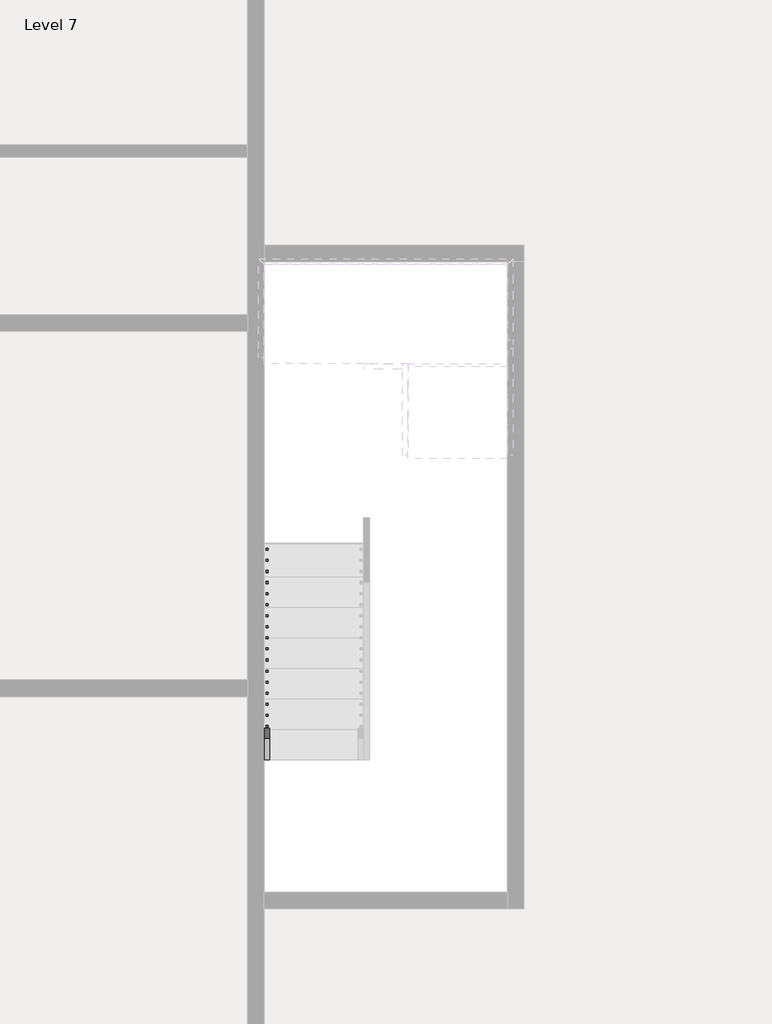
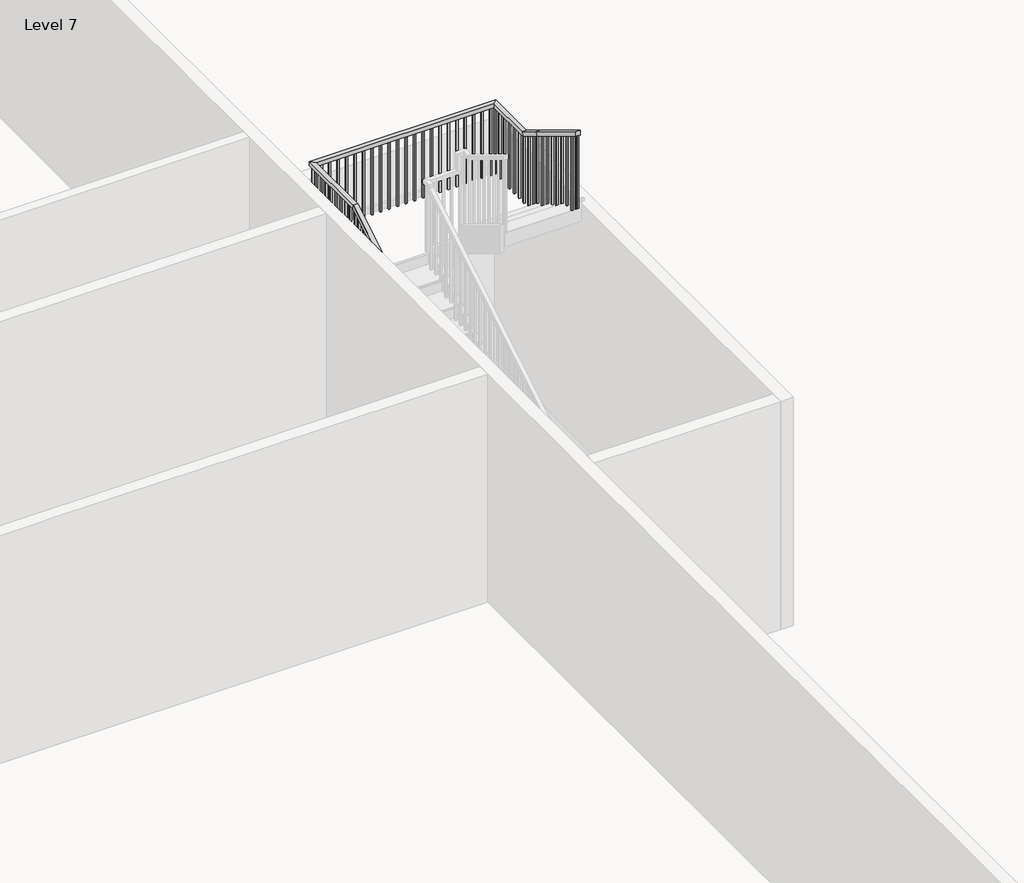
# One storey, part 6 of 8: 1 railing.
"""IFC4 building model written with IfcOpenShell, lengths in millimetres."""

from ifc_helpers import new_model, si_unit, frame, origin, place, context, project, spatial, polyline, outline, extrude, faceted_brep, element, save

model = new_model("IFC4")

# Units and contexts
model_context = context("Model", 3, world=origin())
ifc_project = project(units=[si_unit("LENGTHUNIT", "METRE", prefix="MILLI")], contexts=[model_context])

# Site, building, storey
site = spatial("IfcSite", under=ifc_project)
building = spatial("IfcBuilding", under=site)
storey = spatial("IfcBuildingStorey", under=building, Name="Level 7", Elevation=43522.6172466)

# Railing
placement = place(None, origin())
element("IfcRailing", 1, ObjectType="Handrail - Rectangular", at=placement, inside=storey, context=model_context, shape_type="SolidModel", body=[
    faceted_brep([(-3617.4415084, -23154.3851539, 44606.3505799), (-3617.4415084, -23154.3851539, 44546.9491197), (-3566.6415084, -23154.3851539, 44546.9491197), (-3566.6415084, -23154.3851539, 44606.3505799), (-3617.4415084, -19522.1851539, 46807.6839133), (-3617.4415084, -19507.9927445, 46756.8839133), (-3566.6415084, -19507.9927445, 46756.8839133), (-3566.6415084, -19522.1851539, 46807.6839133), (-3617.4415084, -18607.7851539, 46807.6839133), (-3617.4415084, -18607.7851539, 46756.8839133), (-3566.6415084, -18658.5851539, 46756.8839133), (-3566.6415084, -18658.5851539, 46807.6839133), (-1382.2415084, -18607.7851539, 46807.6839133), (-1382.2415084, -18607.7851539, 46756.8839133), (-1433.0415084, -18658.5851539, 46756.8839133), (-1433.0415084, -18658.5851539, 46807.6839133), (-1382.2415084, -19242.7851539, 46807.6839133), (-1382.2415084, -19256.9775633, 46756.8839133), (-1433.0415084, -19256.9775633, 46756.8839133), (-1433.0415084, -19242.7851539, 46807.6839133), (-1382.2415084, -19522.1851539, 46977.0172466), (-1382.2415084, -19548.5148811, 46933.5731968), (-1433.0415084, -19548.5148811, 46933.5731968), (-1433.0415084, -19522.1851539, 46977.0172466), (-1382.2415084, -20360.3851539, 47485.0172466), (-1433.0415084, -20360.3851539, 47485.0172466), (-1433.0415084, -20360.3851539, 47425.6157863), (-1382.2415084, -20360.3851539, 47425.6157863)], [[[0, 1, 2, 3]], [[1, 0, 4, 5]], [[2, 1, 5, 6]], [[3, 2, 6, 7]], [[0, 3, 7, 4]], [[5, 4, 8, 9]], [[6, 5, 9, 10]], [[7, 6, 10, 11]], [[4, 7, 11, 8]], [[9, 8, 12, 13]], [[10, 9, 13, 14]], [[11, 10, 14, 15]], [[8, 11, 15, 12]], [[13, 12, 16, 17]], [[14, 13, 17, 18]], [[15, 14, 18, 19]], [[12, 15, 19, 16]], [[17, 16, 20, 21]], [[18, 17, 21, 22]], [[19, 18, 22, 23]], [[16, 19, 23, 20]], [[24, 25, 26, 27]], [[21, 20, 24, 27]], [[22, 21, 27, 26]], [[23, 22, 26, 25]], [[20, 23, 25, 24]]]),
    extrude(outline(polyline([(-20325.4601539, 47404.4491197), (-20325.4601539, 46401.2839133), (-20344.5101539, 46401.2839133), (-20344.5101539, 47415.9945742), (-20325.4601539, 47404.4491197)])), frame((-1417.1665084, 0.0, 0.0), z_axis=(1.0, 0.0, 0.0), x_axis=(0.0, 1.0, 0.0)), (0.0, 0.0, 1.0), 19.05),
    extrude(outline(polyline([(-20223.8601539, 47342.8733621), (-20223.8601539, 46401.2839133), (-20242.9101539, 46401.2839133), (-20242.9101539, 47354.4188166), (-20223.8601539, 47342.8733621)])), frame((-1417.1665084, 0.0, 0.0), z_axis=(1.0, 0.0, 0.0), x_axis=(0.0, 1.0, 0.0)), (0.0, 0.0, 1.0), 19.05),
    extrude(outline(polyline([(-20122.2601539, 47281.2976045), (-20122.2601539, 46401.2839133), (-20141.3101539, 46401.2839133), (-20141.3101539, 47292.8430591), (-20122.2601539, 47281.2976045)])), frame((-1417.1665084, 0.0, 0.0), z_axis=(1.0, 0.0, 0.0), x_axis=(0.0, 1.0, 0.0)), (0.0, 0.0, 1.0), 19.05),
    extrude(outline(polyline([(-20020.6601539, 47219.721847), (-20020.6601539, 46231.9505799), (-20039.7101539, 46231.9505799), (-20039.7101539, 47231.2673015), (-20020.6601539, 47219.721847)])), frame((-1417.1665084, 0.0, 0.0), z_axis=(1.0, 0.0, 0.0), x_axis=(0.0, 1.0, 0.0)), (0.0, 0.0, 1.0), 19.05),
    extrude(outline(polyline([(-19919.0601539, 47158.1460894), (-19919.0601539, 46231.9505799), (-19938.1101539, 46231.9505799), (-19938.1101539, 47169.6915439), (-19919.0601539, 47158.1460894)])), frame((-1417.1665084, 0.0, 0.0), z_axis=(1.0, 0.0, 0.0), x_axis=(0.0, 1.0, 0.0)), (0.0, 0.0, 1.0), 19.05),
    extrude(outline(polyline([(-19817.4601539, 47096.5703318), (-19817.4601539, 46231.9505799), (-19836.5101539, 46231.9505799), (-19836.5101539, 47108.1157863), (-19817.4601539, 47096.5703318)])), frame((-1417.1665084, 0.0, 0.0), z_axis=(1.0, 0.0, 0.0), x_axis=(0.0, 1.0, 0.0)), (0.0, 0.0, 1.0), 19.05),
    extrude(outline(polyline([(-19715.8601539, 47034.9945742), (-19715.8601539, 46062.6172466), (-19734.9101539, 46062.6172466), (-19734.9101539, 47046.5400288), (-19715.8601539, 47034.9945742)])), frame((-1417.1665084, 0.0, 0.0), z_axis=(1.0, 0.0, 0.0), x_axis=(0.0, 1.0, 0.0)), (0.0, 0.0, 1.0), 19.05),
    extrude(outline(polyline([(-19614.2601539, 46973.4188166), (-19614.2601539, 46062.6172466), (-19633.3101539, 46062.6172466), (-19633.3101539, 46984.9642712), (-19614.2601539, 46973.4188166)])), frame((-1417.1665084, 0.0, 0.0), z_axis=(1.0, 0.0, 0.0), x_axis=(0.0, 1.0, 0.0)), (0.0, 0.0, 1.0), 19.05),
    extrude(outline(polyline([(-19436.4601539, 46865.6612409), (-19436.4601539, 45893.2839133), (-19455.5101539, 45893.2839133), (-19455.5101539, 46877.2066954), (-19436.4601539, 46865.6612409)])), frame((-1417.1665084, 0.0, 0.0), z_axis=(1.0, 0.0, 0.0), x_axis=(0.0, 1.0, 0.0)), (0.0, 0.0, 1.0), 19.05),
    extrude(outline(polyline([(-19334.8601539, 46804.0854833), (-19334.8601539, 45893.2839133), (-19353.9101539, 45893.2839133), (-19353.9101539, 46815.6309379), (-19334.8601539, 46804.0854833)])), frame((-1417.1665084, 0.0, 0.0), z_axis=(1.0, 0.0, 0.0), x_axis=(0.0, 1.0, 0.0)), (0.0, 0.0, 1.0), 19.05),
    extrude(outline(polyline([(-1398.1165084, -19233.2601539), (-1398.1165084, -19252.3101539), (-1417.1665084, -19252.3101539), (-1417.1665084, -19233.2601539), (-1398.1165084, -19233.2601539)])), frame((0.0, 0.0, 45893.2839133), z_axis=(0.0, 0.0, 1.0), x_axis=(1.0, 0.0, 0.0)), (0.0, 0.0, 1.0), 863.6),
    extrude(outline(polyline([(-1398.1165084, -19131.6601539), (-1398.1165084, -19150.7101539), (-1417.1665084, -19150.7101539), (-1417.1665084, -19131.6601539), (-1398.1165084, -19131.6601539)])), frame((0.0, 0.0, 45893.2839133), z_axis=(0.0, 0.0, 1.0), x_axis=(1.0, 0.0, 0.0)), (0.0, 0.0, 1.0), 863.6),
    extrude(outline(polyline([(-1398.1165084, -19030.0601539), (-1398.1165084, -19049.1101539), (-1417.1665084, -19049.1101539), (-1417.1665084, -19030.0601539), (-1398.1165084, -19030.0601539)])), frame((0.0, 0.0, 45893.2839133), z_axis=(0.0, 0.0, 1.0), x_axis=(1.0, 0.0, 0.0)), (0.0, 0.0, 1.0), 863.6),
    extrude(outline(polyline([(-1398.1165084, -18928.4601539), (-1398.1165084, -18947.5101539), (-1417.1665084, -18947.5101539), (-1417.1665084, -18928.4601539), (-1398.1165084, -18928.4601539)])), frame((0.0, 0.0, 45893.2839133), z_axis=(0.0, 0.0, 1.0), x_axis=(1.0, 0.0, 0.0)), (0.0, 0.0, 1.0), 863.6),
    extrude(outline(polyline([(-1398.1165084, -18826.8601539), (-1398.1165084, -18845.9101539), (-1417.1665084, -18845.9101539), (-1417.1665084, -18826.8601539), (-1398.1165084, -18826.8601539)])), frame((0.0, 0.0, 45893.2839133), z_axis=(0.0, 0.0, 1.0), x_axis=(1.0, 0.0, 0.0)), (0.0, 0.0, 1.0), 863.6),
    extrude(outline(polyline([(-1398.1165084, -18725.2601539), (-1398.1165084, -18744.3101539), (-1417.1665084, -18744.3101539), (-1417.1665084, -18725.2601539), (-1398.1165084, -18725.2601539)])), frame((0.0, 0.0, 45893.2839133), z_axis=(0.0, 0.0, 1.0), x_axis=(1.0, 0.0, 0.0)), (0.0, 0.0, 1.0), 863.6),
    extrude(outline(polyline([(-1467.9665084, -18623.6601539), (-1448.9165084, -18623.6601539), (-1448.9165084, -18642.7101539), (-1467.9665084, -18642.7101539), (-1467.9665084, -18623.6601539)])), frame((0.0, 0.0, 45893.2839133), z_axis=(0.0, 0.0, 1.0), x_axis=(1.0, 0.0, 0.0)), (0.0, 0.0, 1.0), 863.6),
    extrude(outline(polyline([(-1569.5665084, -18623.6601539), (-1550.5165084, -18623.6601539), (-1550.5165084, -18642.7101539), (-1569.5665084, -18642.7101539), (-1569.5665084, -18623.6601539)])), frame((0.0, 0.0, 45893.2839133), z_axis=(0.0, 0.0, 1.0), x_axis=(1.0, 0.0, 0.0)), (0.0, 0.0, 1.0), 863.6),
    extrude(outline(polyline([(-1671.1665084, -18623.6601539), (-1652.1165084, -18623.6601539), (-1652.1165084, -18642.7101539), (-1671.1665084, -18642.7101539), (-1671.1665084, -18623.6601539)])), frame((0.0, 0.0, 45893.2839133), z_axis=(0.0, 0.0, 1.0), x_axis=(1.0, 0.0, 0.0)), (0.0, 0.0, 1.0), 863.6),
    extrude(outline(polyline([(-1772.7665084, -18623.6601539), (-1753.7165084, -18623.6601539), (-1753.7165084, -18642.7101539), (-1772.7665084, -18642.7101539), (-1772.7665084, -18623.6601539)])), frame((0.0, 0.0, 45893.2839133), z_axis=(0.0, 0.0, 1.0), x_axis=(1.0, 0.0, 0.0)), (0.0, 0.0, 1.0), 863.6),
    extrude(outline(polyline([(-1874.3665084, -18623.6601539), (-1855.3165084, -18623.6601539), (-1855.3165084, -18642.7101539), (-1874.3665084, -18642.7101539), (-1874.3665084, -18623.6601539)])), frame((0.0, 0.0, 45893.2839133), z_axis=(0.0, 0.0, 1.0), x_axis=(1.0, 0.0, 0.0)), (0.0, 0.0, 1.0), 863.6),
    extrude(outline(polyline([(-1975.9665084, -18623.6601539), (-1956.9165084, -18623.6601539), (-1956.9165084, -18642.7101539), (-1975.9665084, -18642.7101539), (-1975.9665084, -18623.6601539)])), frame((0.0, 0.0, 45893.2839133), z_axis=(0.0, 0.0, 1.0), x_axis=(1.0, 0.0, 0.0)), (0.0, 0.0, 1.0), 863.6),
    extrude(outline(polyline([(-2077.5665084, -18623.6601539), (-2058.5165084, -18623.6601539), (-2058.5165084, -18642.7101539), (-2077.5665084, -18642.7101539), (-2077.5665084, -18623.6601539)])), frame((0.0, 0.0, 45893.2839133), z_axis=(0.0, 0.0, 1.0), x_axis=(1.0, 0.0, 0.0)), (0.0, 0.0, 1.0), 863.6),
    extrude(outline(polyline([(-2179.1665084, -18623.6601539), (-2160.1165084, -18623.6601539), (-2160.1165084, -18642.7101539), (-2179.1665084, -18642.7101539), (-2179.1665084, -18623.6601539)])), frame((0.0, 0.0, 45893.2839133), z_axis=(0.0, 0.0, 1.0), x_axis=(1.0, 0.0, 0.0)), (0.0, 0.0, 1.0), 863.6),
    extrude(outline(polyline([(-2280.7665084, -18623.6601539), (-2261.7165084, -18623.6601539), (-2261.7165084, -18642.7101539), (-2280.7665084, -18642.7101539), (-2280.7665084, -18623.6601539)])), frame((0.0, 0.0, 45893.2839133), z_axis=(0.0, 0.0, 1.0), x_axis=(1.0, 0.0, 0.0)), (0.0, 0.0, 1.0), 863.6),
    extrude(outline(polyline([(-2382.3665084, -18623.6601539), (-2363.3165084, -18623.6601539), (-2363.3165084, -18642.7101539), (-2382.3665084, -18642.7101539), (-2382.3665084, -18623.6601539)])), frame((0.0, 0.0, 45893.2839133), z_axis=(0.0, 0.0, 1.0), x_axis=(1.0, 0.0, 0.0)), (0.0, 0.0, 1.0), 863.6),
    extrude(outline(polyline([(-2483.9665084, -18623.6601539), (-2464.9165084, -18623.6601539), (-2464.9165084, -18642.7101539), (-2483.9665084, -18642.7101539), (-2483.9665084, -18623.6601539)])), frame((0.0, 0.0, 45893.2839133), z_axis=(0.0, 0.0, 1.0), x_axis=(1.0, 0.0, 0.0)), (0.0, 0.0, 1.0), 863.6),
    extrude(outline(polyline([(-2585.5665084, -18623.6601539), (-2566.5165084, -18623.6601539), (-2566.5165084, -18642.7101539), (-2585.5665084, -18642.7101539), (-2585.5665084, -18623.6601539)])), frame((0.0, 0.0, 45893.2839133), z_axis=(0.0, 0.0, 1.0), x_axis=(1.0, 0.0, 0.0)), (0.0, 0.0, 1.0), 863.6),
    extrude(outline(polyline([(-2687.1665084, -18623.6601539), (-2668.1165084, -18623.6601539), (-2668.1165084, -18642.7101539), (-2687.1665084, -18642.7101539), (-2687.1665084, -18623.6601539)])), frame((0.0, 0.0, 45893.2839133), z_axis=(0.0, 0.0, 1.0), x_axis=(1.0, 0.0, 0.0)), (0.0, 0.0, 1.0), 863.6),
    extrude(outline(polyline([(-2788.7665084, -18623.6601539), (-2769.7165084, -18623.6601539), (-2769.7165084, -18642.7101539), (-2788.7665084, -18642.7101539), (-2788.7665084, -18623.6601539)])), frame((0.0, 0.0, 45893.2839133), z_axis=(0.0, 0.0, 1.0), x_axis=(1.0, 0.0, 0.0)), (0.0, 0.0, 1.0), 863.6),
    extrude(outline(polyline([(-2890.3665084, -18623.6601539), (-2871.3165084, -18623.6601539), (-2871.3165084, -18642.7101539), (-2890.3665084, -18642.7101539), (-2890.3665084, -18623.6601539)])), frame((0.0, 0.0, 45893.2839133), z_axis=(0.0, 0.0, 1.0), x_axis=(1.0, 0.0, 0.0)), (0.0, 0.0, 1.0), 863.6),
    extrude(outline(polyline([(-2991.9665084, -18623.6601539), (-2972.9165084, -18623.6601539), (-2972.9165084, -18642.7101539), (-2991.9665084, -18642.7101539), (-2991.9665084, -18623.6601539)])), frame((0.0, 0.0, 45893.2839133), z_axis=(0.0, 0.0, 1.0), x_axis=(1.0, 0.0, 0.0)), (0.0, 0.0, 1.0), 863.6),
    extrude(outline(polyline([(-3093.5665084, -18623.6601539), (-3074.5165084, -18623.6601539), (-3074.5165084, -18642.7101539), (-3093.5665084, -18642.7101539), (-3093.5665084, -18623.6601539)])), frame((0.0, 0.0, 45893.2839133), z_axis=(0.0, 0.0, 1.0), x_axis=(1.0, 0.0, 0.0)), (0.0, 0.0, 1.0), 863.6),
    extrude(outline(polyline([(-3195.1665084, -18623.6601539), (-3176.1165084, -18623.6601539), (-3176.1165084, -18642.7101539), (-3195.1665084, -18642.7101539), (-3195.1665084, -18623.6601539)])), frame((0.0, 0.0, 45893.2839133), z_axis=(0.0, 0.0, 1.0), x_axis=(1.0, 0.0, 0.0)), (0.0, 0.0, 1.0), 863.6),
    extrude(outline(polyline([(-3296.7665084, -18623.6601539), (-3277.7165084, -18623.6601539), (-3277.7165084, -18642.7101539), (-3296.7665084, -18642.7101539), (-3296.7665084, -18623.6601539)])), frame((0.0, 0.0, 45893.2839133), z_axis=(0.0, 0.0, 1.0), x_axis=(1.0, 0.0, 0.0)), (0.0, 0.0, 1.0), 863.6),
    extrude(outline(polyline([(-3398.3665084, -18623.6601539), (-3379.3165084, -18623.6601539), (-3379.3165084, -18642.7101539), (-3398.3665084, -18642.7101539), (-3398.3665084, -18623.6601539)])), frame((0.0, 0.0, 45893.2839133), z_axis=(0.0, 0.0, 1.0), x_axis=(1.0, 0.0, 0.0)), (0.0, 0.0, 1.0), 863.6),
    extrude(outline(polyline([(-3499.9665084, -18623.6601539), (-3480.9165084, -18623.6601539), (-3480.9165084, -18642.7101539), (-3499.9665084, -18642.7101539), (-3499.9665084, -18623.6601539)])), frame((0.0, 0.0, 45893.2839133), z_axis=(0.0, 0.0, 1.0), x_axis=(1.0, 0.0, 0.0)), (0.0, 0.0, 1.0), 863.6),
    extrude(outline(polyline([(-3601.5665084, -18718.9101539), (-3601.5665084, -18699.8601539), (-3582.5165084, -18699.8601539), (-3582.5165084, -18718.9101539), (-3601.5665084, -18718.9101539)])), frame((0.0, 0.0, 45893.2839133), z_axis=(0.0, 0.0, 1.0), x_axis=(1.0, 0.0, 0.0)), (0.0, 0.0, 1.0), 863.6),
    extrude(outline(polyline([(-3601.5665084, -18820.5101539), (-3601.5665084, -18801.4601539), (-3582.5165084, -18801.4601539), (-3582.5165084, -18820.5101539), (-3601.5665084, -18820.5101539)])), frame((0.0, 0.0, 45893.2839133), z_axis=(0.0, 0.0, 1.0), x_axis=(1.0, 0.0, 0.0)), (0.0, 0.0, 1.0), 863.6),
    extrude(outline(polyline([(-3601.5665084, -18922.1101539), (-3601.5665084, -18903.0601539), (-3582.5165084, -18903.0601539), (-3582.5165084, -18922.1101539), (-3601.5665084, -18922.1101539)])), frame((0.0, 0.0, 45893.2839133), z_axis=(0.0, 0.0, 1.0), x_axis=(1.0, 0.0, 0.0)), (0.0, 0.0, 1.0), 863.6),
    extrude(outline(polyline([(-3601.5665084, -19023.7101539), (-3601.5665084, -19004.6601539), (-3582.5165084, -19004.6601539), (-3582.5165084, -19023.7101539), (-3601.5665084, -19023.7101539)])), frame((0.0, 0.0, 45893.2839133), z_axis=(0.0, 0.0, 1.0), x_axis=(1.0, 0.0, 0.0)), (0.0, 0.0, 1.0), 863.6),
    extrude(outline(polyline([(-3601.5665084, -19125.3101539), (-3601.5665084, -19106.2601539), (-3582.5165084, -19106.2601539), (-3582.5165084, -19125.3101539), (-3601.5665084, -19125.3101539)])), frame((0.0, 0.0, 45893.2839133), z_axis=(0.0, 0.0, 1.0), x_axis=(1.0, 0.0, 0.0)), (0.0, 0.0, 1.0), 863.6),
    extrude(outline(polyline([(-3601.5665084, -19226.9101539), (-3601.5665084, -19207.8601539), (-3582.5165084, -19207.8601539), (-3582.5165084, -19226.9101539), (-3601.5665084, -19226.9101539)])), frame((0.0, 0.0, 45893.2839133), z_axis=(0.0, 0.0, 1.0), x_axis=(1.0, 0.0, 0.0)), (0.0, 0.0, 1.0), 863.6),
    extrude(outline(polyline([(-3601.5665084, -19328.5101539), (-3601.5665084, -19309.4601539), (-3582.5165084, -19309.4601539), (-3582.5165084, -19328.5101539), (-3601.5665084, -19328.5101539)])), frame((0.0, 0.0, 45893.2839133), z_axis=(0.0, 0.0, 1.0), x_axis=(1.0, 0.0, 0.0)), (0.0, 0.0, 1.0), 863.6),
    extrude(outline(polyline([(-3601.5665084, -19430.1101539), (-3601.5665084, -19411.0601539), (-3582.5165084, -19411.0601539), (-3582.5165084, -19430.1101539), (-3601.5665084, -19430.1101539)])), frame((0.0, 0.0, 45893.2839133), z_axis=(0.0, 0.0, 1.0), x_axis=(1.0, 0.0, 0.0)), (0.0, 0.0, 1.0), 863.6),
    extrude(outline(polyline([(-19588.8601539, 46707.8733621), (-19588.8601539, 45723.9505799), (-19607.9101539, 45723.9505799), (-19607.9101539, 46696.3279076), (-19588.8601539, 46707.8733621)])), frame((-3601.5665084, 0.0, 0.0), z_axis=(1.0, 0.0, 0.0), x_axis=(0.0, 1.0, 0.0)), (0.0, 0.0, 1.0), 19.05),
    extrude(outline(polyline([(-19690.4601539, 46646.2976045), (-19690.4601539, 45723.9505799), (-19709.5101539, 45723.9505799), (-19709.5101539, 46634.75215), (-19690.4601539, 46646.2976045)])), frame((-3601.5665084, 0.0, 0.0), z_axis=(1.0, 0.0, 0.0), x_axis=(0.0, 1.0, 0.0)), (0.0, 0.0, 1.0), 19.05),
    extrude(outline(polyline([(-19792.0601539, 46584.721847), (-19792.0601539, 45723.9505799), (-19811.1101539, 45723.9505799), (-19811.1101539, 46573.1763924), (-19792.0601539, 46584.721847)])), frame((-3601.5665084, 0.0, 0.0), z_axis=(1.0, 0.0, 0.0), x_axis=(0.0, 1.0, 0.0)), (0.0, 0.0, 1.0), 19.05),
    extrude(outline(polyline([(-19893.6601539, 46523.1460894), (-19893.6601539, 45554.6172466), (-19912.7101539, 45554.6172466), (-19912.7101539, 46511.6006348), (-19893.6601539, 46523.1460894)])), frame((-3601.5665084, 0.0, 0.0), z_axis=(1.0, 0.0, 0.0), x_axis=(0.0, 1.0, 0.0)), (0.0, 0.0, 1.0), 19.05),
    extrude(outline(polyline([(-19995.2601539, 46461.5703318), (-19995.2601539, 45554.6172466), (-20014.3101539, 45554.6172466), (-20014.3101539, 46450.0248773), (-19995.2601539, 46461.5703318)])), frame((-3601.5665084, 0.0, 0.0), z_axis=(1.0, 0.0, 0.0), x_axis=(0.0, 1.0, 0.0)), (0.0, 0.0, 1.0), 19.05),
    extrude(outline(polyline([(-20096.8601539, 46399.9945742), (-20096.8601539, 45385.2839133), (-20115.9101539, 45385.2839133), (-20115.9101539, 46388.4491197), (-20096.8601539, 46399.9945742)])), frame((-3601.5665084, 0.0, 0.0), z_axis=(1.0, 0.0, 0.0), x_axis=(0.0, 1.0, 0.0)), (0.0, 0.0, 1.0), 19.05),
    extrude(outline(polyline([(-20198.4601539, 46338.4188166), (-20198.4601539, 45385.2839133), (-20217.5101539, 45385.2839133), (-20217.5101539, 46326.8733621), (-20198.4601539, 46338.4188166)])), frame((-3601.5665084, 0.0, 0.0), z_axis=(1.0, 0.0, 0.0), x_axis=(0.0, 1.0, 0.0)), (0.0, 0.0, 1.0), 19.05),
    extrude(outline(polyline([(-20300.0601539, 46276.8430591), (-20300.0601539, 45385.2839133), (-20319.1101539, 45385.2839133), (-20319.1101539, 46265.2976045), (-20300.0601539, 46276.8430591)])), frame((-3601.5665084, 0.0, 0.0), z_axis=(1.0, 0.0, 0.0), x_axis=(0.0, 1.0, 0.0)), (0.0, 0.0, 1.0), 19.05),
    extrude(outline(polyline([(-20401.6601539, 46215.2673015), (-20401.6601539, 45215.9505799), (-20420.7101539, 45215.9505799), (-20420.7101539, 46203.721847), (-20401.6601539, 46215.2673015)])), frame((-3601.5665084, 0.0, 0.0), z_axis=(1.0, 0.0, 0.0), x_axis=(0.0, 1.0, 0.0)), (0.0, 0.0, 1.0), 19.05),
    extrude(outline(polyline([(-20503.2601539, 46153.6915439), (-20503.2601539, 45215.9505799), (-20522.3101539, 45215.9505799), (-20522.3101539, 46142.1460894), (-20503.2601539, 46153.6915439)])), frame((-3601.5665084, 0.0, 0.0), z_axis=(1.0, 0.0, 0.0), x_axis=(0.0, 1.0, 0.0)), (0.0, 0.0, 1.0), 19.05),
    extrude(outline(polyline([(-20604.8601539, 46092.1157863), (-20604.8601539, 45215.9505799), (-20623.9101539, 45215.9505799), (-20623.9101539, 46080.5703318), (-20604.8601539, 46092.1157863)])), frame((-3601.5665084, 0.0, 0.0), z_axis=(1.0, 0.0, 0.0), x_axis=(0.0, 1.0, 0.0)), (0.0, 0.0, 1.0), 19.05),
    extrude(outline(polyline([(-20706.4601539, 46030.5400288), (-20706.4601539, 45046.6172466), (-20725.5101539, 45046.6172466), (-20725.5101539, 46018.9945742), (-20706.4601539, 46030.5400288)])), frame((-3601.5665084, 0.0, 0.0), z_axis=(1.0, 0.0, 0.0), x_axis=(0.0, 1.0, 0.0)), (0.0, 0.0, 1.0), 19.05),
    extrude(outline(polyline([(-20808.0601539, 45968.9642712), (-20808.0601539, 45046.6172466), (-20827.1101539, 45046.6172466), (-20827.1101539, 45957.4188166), (-20808.0601539, 45968.9642712)])), frame((-3601.5665084, 0.0, 0.0), z_axis=(1.0, 0.0, 0.0), x_axis=(0.0, 1.0, 0.0)), (0.0, 0.0, 1.0), 19.05),
    extrude(outline(polyline([(-20909.6601539, 45907.3885136), (-20909.6601539, 45046.6172466), (-20928.7101539, 45046.6172466), (-20928.7101539, 45895.8430591), (-20909.6601539, 45907.3885136)])), frame((-3601.5665084, 0.0, 0.0), z_axis=(1.0, 0.0, 0.0), x_axis=(0.0, 1.0, 0.0)), (0.0, 0.0, 1.0), 19.05),
    extrude(outline(polyline([(-21011.2601539, 45845.812756), (-21011.2601539, 44877.2839133), (-21030.3101539, 44877.2839133), (-21030.3101539, 45834.2673015), (-21011.2601539, 45845.812756)])), frame((-3601.5665084, 0.0, 0.0), z_axis=(1.0, 0.0, 0.0), x_axis=(0.0, 1.0, 0.0)), (0.0, 0.0, 1.0), 19.05),
    extrude(outline(polyline([(-21112.8601539, 45784.2369985), (-21112.8601539, 44877.2839133), (-21131.9101539, 44877.2839133), (-21131.9101539, 45772.6915439), (-21112.8601539, 45784.2369985)])), frame((-3601.5665084, 0.0, 0.0), z_axis=(1.0, 0.0, 0.0), x_axis=(0.0, 1.0, 0.0)), (0.0, 0.0, 1.0), 19.05),
    extrude(outline(polyline([(-21214.4601539, 45722.6612409), (-21214.4601539, 44707.9505799), (-21233.5101539, 44707.9505799), (-21233.5101539, 45711.1157863), (-21214.4601539, 45722.6612409)])), frame((-3601.5665084, 0.0, 0.0), z_axis=(1.0, 0.0, 0.0), x_axis=(0.0, 1.0, 0.0)), (0.0, 0.0, 1.0), 19.05),
    extrude(outline(polyline([(-21316.0601539, 45661.0854833), (-21316.0601539, 44707.9505799), (-21335.1101539, 44707.9505799), (-21335.1101539, 45649.5400288), (-21316.0601539, 45661.0854833)])), frame((-3601.5665084, 0.0, 0.0), z_axis=(1.0, 0.0, 0.0), x_axis=(0.0, 1.0, 0.0)), (0.0, 0.0, 1.0), 19.05),
    extrude(outline(polyline([(-21417.6601539, 45599.5097257), (-21417.6601539, 44707.9505799), (-21436.7101539, 44707.9505799), (-21436.7101539, 45587.9642712), (-21417.6601539, 45599.5097257)])), frame((-3601.5665084, 0.0, 0.0), z_axis=(1.0, 0.0, 0.0), x_axis=(0.0, 1.0, 0.0)), (0.0, 0.0, 1.0), 19.05),
    extrude(outline(polyline([(-21519.2601539, 45537.9339682), (-21519.2601539, 44538.6172466), (-21538.3101539, 44538.6172466), (-21538.3101539, 45526.3885136), (-21519.2601539, 45537.9339682)])), frame((-3601.5665084, 0.0, 0.0), z_axis=(1.0, 0.0, 0.0), x_axis=(0.0, 1.0, 0.0)), (0.0, 0.0, 1.0), 19.05),
    extrude(outline(polyline([(-21620.8601539, 45476.3582106), (-21620.8601539, 44538.6172466), (-21639.9101539, 44538.6172466), (-21639.9101539, 45464.812756), (-21620.8601539, 45476.3582106)])), frame((-3601.5665084, 0.0, 0.0), z_axis=(1.0, 0.0, 0.0), x_axis=(0.0, 1.0, 0.0)), (0.0, 0.0, 1.0), 19.05),
    extrude(outline(polyline([(-21722.4601539, 45414.782453), (-21722.4601539, 44538.6172466), (-21741.5101539, 44538.6172466), (-21741.5101539, 45403.2369985), (-21722.4601539, 45414.782453)])), frame((-3601.5665084, 0.0, 0.0), z_axis=(1.0, 0.0, 0.0), x_axis=(0.0, 1.0, 0.0)), (0.0, 0.0, 1.0), 19.05),
    extrude(outline(polyline([(-21824.0601539, 45353.2066954), (-21824.0601539, 44369.2839133), (-21843.1101539, 44369.2839133), (-21843.1101539, 45341.6612409), (-21824.0601539, 45353.2066954)])), frame((-3601.5665084, 0.0, 0.0), z_axis=(1.0, 0.0, 0.0), x_axis=(0.0, 1.0, 0.0)), (0.0, 0.0, 1.0), 19.05),
    extrude(outline(polyline([(-21925.6601539, 45291.6309379), (-21925.6601539, 44369.2839133), (-21944.7101539, 44369.2839133), (-21944.7101539, 45280.0854833), (-21925.6601539, 45291.6309379)])), frame((-3601.5665084, 0.0, 0.0), z_axis=(1.0, 0.0, 0.0), x_axis=(0.0, 1.0, 0.0)), (0.0, 0.0, 1.0), 19.05),
    extrude(outline(polyline([(-22027.2601539, 45230.0551803), (-22027.2601539, 44369.2839133), (-22046.3101539, 44369.2839133), (-22046.3101539, 45218.5097257), (-22027.2601539, 45230.0551803)])), frame((-3601.5665084, 0.0, 0.0), z_axis=(1.0, 0.0, 0.0), x_axis=(0.0, 1.0, 0.0)), (0.0, 0.0, 1.0), 19.05),
    extrude(outline(polyline([(-22128.8601539, 45168.4794227), (-22128.8601539, 44199.9505799), (-22147.9101539, 44199.9505799), (-22147.9101539, 45156.9339682), (-22128.8601539, 45168.4794227)])), frame((-3601.5665084, 0.0, 0.0), z_axis=(1.0, 0.0, 0.0), x_axis=(0.0, 1.0, 0.0)), (0.0, 0.0, 1.0), 19.05),
    extrude(outline(polyline([(-22230.4601539, 45106.9036651), (-22230.4601539, 44199.9505799), (-22249.5101539, 44199.9505799), (-22249.5101539, 45095.3582106), (-22230.4601539, 45106.9036651)])), frame((-3601.5665084, 0.0, 0.0), z_axis=(1.0, 0.0, 0.0), x_axis=(0.0, 1.0, 0.0)), (0.0, 0.0, 1.0), 19.05),
    extrude(outline(polyline([(-22332.0601539, 45045.3279076), (-22332.0601539, 44030.6172466), (-22351.1101539, 44030.6172466), (-22351.1101539, 45033.782453), (-22332.0601539, 45045.3279076)])), frame((-3601.5665084, 0.0, 0.0), z_axis=(1.0, 0.0, 0.0), x_axis=(0.0, 1.0, 0.0)), (0.0, 0.0, 1.0), 19.05),
    extrude(outline(polyline([(-22433.6601539, 44983.75215), (-22433.6601539, 44030.6172466), (-22452.7101539, 44030.6172466), (-22452.7101539, 44972.2066954), (-22433.6601539, 44983.75215)])), frame((-3601.5665084, 0.0, 0.0), z_axis=(1.0, 0.0, 0.0), x_axis=(0.0, 1.0, 0.0)), (0.0, 0.0, 1.0), 19.05),
    extrude(outline(polyline([(-22535.2601539, 44922.1763924), (-22535.2601539, 44030.6172466), (-22554.3101539, 44030.6172466), (-22554.3101539, 44910.6309379), (-22535.2601539, 44922.1763924)])), frame((-3601.5665084, 0.0, 0.0), z_axis=(1.0, 0.0, 0.0), x_axis=(0.0, 1.0, 0.0)), (0.0, 0.0, 1.0), 19.05),
    extrude(outline(polyline([(-22636.8601539, 44860.6006348), (-22636.8601539, 43861.2839133), (-22655.9101539, 43861.2839133), (-22655.9101539, 44849.0551803), (-22636.8601539, 44860.6006348)])), frame((-3601.5665084, 0.0, 0.0), z_axis=(1.0, 0.0, 0.0), x_axis=(0.0, 1.0, 0.0)), (0.0, 0.0, 1.0), 19.05),
    extrude(outline(polyline([(-22738.4601539, 44799.0248773), (-22738.4601539, 43861.2839133), (-22757.5101539, 43861.2839133), (-22757.5101539, 44787.4794227), (-22738.4601539, 44799.0248773)])), frame((-3601.5665084, 0.0, 0.0), z_axis=(1.0, 0.0, 0.0), x_axis=(0.0, 1.0, 0.0)), (0.0, 0.0, 1.0), 19.05),
    extrude(outline(polyline([(-22840.0601539, 44737.4491197), (-22840.0601539, 43861.2839133), (-22859.1101539, 43861.2839133), (-22859.1101539, 44725.9036651), (-22840.0601539, 44737.4491197)])), frame((-3601.5665084, 0.0, 0.0), z_axis=(1.0, 0.0, 0.0), x_axis=(0.0, 1.0, 0.0)), (0.0, 0.0, 1.0), 19.05),
    extrude(outline(polyline([(-22941.6601539, 44675.8733621), (-22941.6601539, 43691.9505799), (-22960.7101539, 43691.9505799), (-22960.7101539, 44664.3279076), (-22941.6601539, 44675.8733621)])), frame((-3601.5665084, 0.0, 0.0), z_axis=(1.0, 0.0, 0.0), x_axis=(0.0, 1.0, 0.0)), (0.0, 0.0, 1.0), 19.05),
    extrude(outline(polyline([(-23043.2601539, 44614.2976045), (-23043.2601539, 43691.9505799), (-23062.3101539, 43691.9505799), (-23062.3101539, 44602.75215), (-23043.2601539, 44614.2976045)])), frame((-3601.5665084, 0.0, 0.0), z_axis=(1.0, 0.0, 0.0), x_axis=(0.0, 1.0, 0.0)), (0.0, 0.0, 1.0), 19.05),
    extrude(outline(polyline([(-19512.6601539, 46911.8430591), (-19512.6601539, 45893.2839133), (-19531.7101539, 45893.2839133), (-19531.7101539, 46923.3885136), (-19512.6601539, 46911.8430591)])), frame((-1417.1665084, 0.0, 0.0), z_axis=(1.0, 0.0, 0.0), x_axis=(0.0, 1.0, 0.0)), (0.0, 0.0, 1.0), 19.05),
    extrude(outline(polyline([(-1417.1665084, -18623.6601539), (-1398.1165084, -18623.6601539), (-1398.1165084, -18642.7101539), (-1417.1665084, -18642.7101539), (-1417.1665084, -18623.6601539)])), frame((0.0, 0.0, 45893.2839133), z_axis=(0.0, 0.0, 1.0), x_axis=(1.0, 0.0, 0.0)), (0.0, 0.0, 1.0), 863.6),
    extrude(outline(polyline([(-3601.5665084, -18642.7101539), (-3601.5665084, -18623.6601539), (-3582.5165084, -18623.6601539), (-3582.5165084, -18642.7101539), (-3601.5665084, -18642.7101539)])), frame((0.0, 0.0, 45893.2839133), z_axis=(0.0, 0.0, 1.0), x_axis=(1.0, 0.0, 0.0)), (0.0, 0.0, 1.0), 863.6),
    extrude(outline(polyline([(-19512.6601539, 46754.0551803), (-19512.6601539, 45893.2839133), (-19531.7101539, 45893.2839133), (-19531.7101539, 46742.5097257), (-19512.6601539, 46754.0551803)])), frame((-3601.5665084, 0.0, 0.0), z_axis=(1.0, 0.0, 0.0), x_axis=(0.0, 1.0, 0.0)), (0.0, 0.0, 1.0), 19.05),
    extrude(outline(polyline([(-20341.3351539, 47414.0703318), (-20341.3351539, 46401.2839133), (-20360.3851539, 46401.2839133), (-20360.3851539, 47425.6157863), (-20341.3351539, 47414.0703318)])), frame((-1417.1665084, 0.0, 0.0), z_axis=(1.0, 0.0, 0.0), x_axis=(0.0, 1.0, 0.0)), (0.0, 0.0, 1.0), 19.05),
    extrude(outline(polyline([(-23135.3351539, 44558.4945742), (-23135.3351539, 43691.9505799), (-23154.3851539, 43691.9505799), (-23154.3851539, 44546.9491197), (-23135.3351539, 44558.4945742)])), frame((-3601.5665084, 0.0, 0.0), z_axis=(1.0, 0.0, 0.0), x_axis=(0.0, 1.0, 0.0)), (0.0, 0.0, 1.0), 19.05),
])

save(model, "model.ifc")

# Revit data of these elements
# Type "Handrail - Rectangular"
#   Assembly Code = "C2010400"
#   built-in parameter 1008612 = 0.0416667 (stored number, unit not read)
#   built-in parameter 1008611 = 0.0416667 (stored number, unit not read)
#   built-in parameter 1008609 = 0.333333 (stored number, unit not read)
#   built-in parameter 1008604 = 0.166667 (stored number, unit not read)
#   built-in parameter 1008603 = 0.166667 (stored number, unit not read)
#   Railing Height = 3' - 0"
#   built-in parameter 1008630 = 2
#   built-in parameter 1008610 = 2
#   built-in parameter 1008618 = Baluster - Square : 3/4"
# Element 1 (IfcRailing, "Handrail - Rectangular")
#   Phase Created = New Construction
